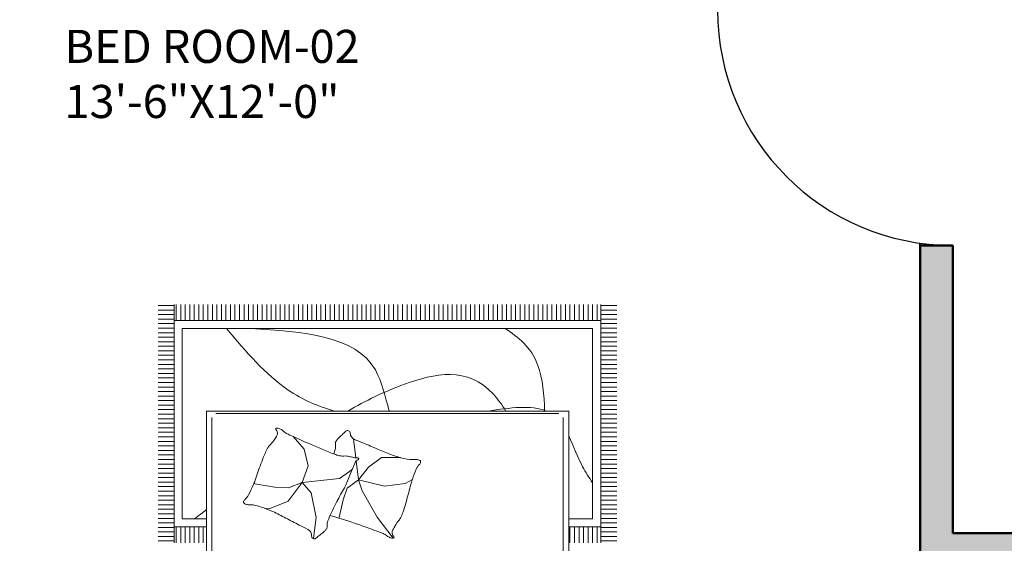
# Model space of a CAD drawing. Units: inches. Extents: x -7 to 1228, y -146 to 1091.
# Tile 22 of 88: x 664 to 815, y 113 to 194. Entities that reach past the tile are written whole.
import ezdxf

# ---------------------------------------------------------------- set-up
doc = ezdxf.new("R2010")
doc.units = ezdxf.units.IN
for name, color, linetype, lineweight in [('A-AREA-IDEN', 7, 'Continuous', 18), ('A-DOOR', 4, 'Continuous', 25), ('A-FURN', 8, 'Continuous', 18), ('A-WALL', 7, 'Continuous', 50), ('A-WALL-PATT', 251, 'Continuous', 13)]:
    doc.layers.add(name, color=color, linetype=linetype, lineweight=lineweight)
doc.styles.add('DIM_FONT', font='SIMPLEX.shx', dxfattribs={"width": 0.8})
doc.styles.get("Standard").update_dxf_attribs({"font": 'arial.ttf'})

# ---------------------------------------------------------------- blocks, each defined once
blk = doc.blocks.new('A$C4F634EDD')
for p, q in [((0.5, 0.5295), (0.5, 2.6295)), ((2.3, 2.6295), (2.3, 0.5295)), ((0.5258, 2.121), (0.5258, 0.5617)), ((2.2716, 0.5617), (2.2716, 1.7136)), ((0.2586, 1.1753), (0.3386, 1.1753)), ((0.3386, 0), (0.3386, 1.1852)), ((0.3486, 1.1052), (0.3486, 1.1852)), ((0.3711, 1.1052), (0.3711, 1.1852)), ((0.3936, 1.1052), (0.3936, 1.1852)), ((0.4161, 1.1052), (0.4161, 1.1852)), ((0.4386, 1.1052), (0.4386, 1.1852)), ((0.4611, 1.1052), (0.4611, 1.1852)), ((0.4836, 1.1052), (0.4836, 1.1852)), ((2.3061, 1.1052), (2.3061, 1.1852)), ((2.3286, 1.1052), (2.3286, 1.1852)), ((2.3511, 1.1052), (2.3511, 1.1852)), ((2.3736, 1.1052), (2.3736, 1.1852)), ((2.3961, 1.1052), (2.3961, 1.1852)), ((2.4186, 1.1052), (2.4186, 1.1852)), ((2.4411, 1.1052), (2.4411, 1.1852)), ((2.4588, 1.1852), (2.4588, 0)), ((2.4588, 1.1753), (2.5388, 1.1753)), ((0.2586, 1.1528), (0.3386, 1.1528)), ((0.2586, 1.1303), (0.3386, 1.1303)), ((1.031, 1.1612), (1.0448, 1.0581)), ((1.4276, 1.1611), (1.3484, 1.0571)), ((2.4588, 1.1528), (2.5388, 1.1528)), ((2.4588, 1.1303), (2.5388, 1.1303)), ((0.2586, 1.1078), (0.3386, 1.1078)), ((0.2586, 1.0853), (0.3386, 1.0853)), ((0.3386, 1.1052), (0.5, 1.1052)), ((2.3, 1.1052), (2.4588, 1.1052)), ((2.4588, 1.1078), (2.5388, 1.1078)), ((2.4588, 1.0853), (2.5388, 1.0853)), ((0.2586, 1.0628), (0.3386, 1.0628)), ((0.2586, 1.0403), (0.3386, 1.0403)), ((0.3786, 1.0652), (0.5, 1.0652)), ((0.3786, 0.12), (0.3786, 1.0652)), ((1.0448, 1.0581), (1.019, 0.936)), ((1.1784, 0.9702), (1.1586, 1.0591)), ((1.3484, 1.0571), (1.2733, 0.9268)), ((2.3, 1.0652), (2.4188, 1.0652)), ((2.4188, 1.0652), (2.4188, 0.12)), ((2.4588, 1.0628), (2.5388, 1.0628)), ((2.4588, 1.0403), (2.5388, 1.0403)), ((0.2586, 1.0178), (0.3386, 1.0178)), ((0.2586, 0.9953), (0.3386, 0.9953)), ((0.8108, 1.0151), (0.7868, 1.0117)), ((0.9054, 0.9773), (0.8108, 1.0151)), ((2.4588, 1.0178), (2.5388, 1.0178)), ((2.4588, 0.9953), (2.5388, 0.9953)), ((0.2586, 0.9728), (0.3386, 0.9728)), ((0.2586, 0.9503), (0.3386, 0.9503)), ((0.9743, 0.8845), (0.9054, 0.9773)), ((1.019, 0.936), (0.9743, 0.8845)), ((1.1982, 0.9129), (1.1784, 0.9702)), ((2.4588, 0.9728), (2.5388, 0.9728)), ((2.4588, 0.9503), (2.5388, 0.9503)), ((0.2586, 0.9278), (0.3386, 0.9278)), ((0.2586, 0.9053), (0.3386, 0.9053)), ((0.2586, 0.8828), (0.3386, 0.8828)), ((0.7403, 0.8913), (0.737, 0.8849)), ((0.8384, 0.9085), (0.7403, 0.8913)), ((0.9072, 0.912), (0.8384, 0.9085)), ((0.9743, 0.8845), (0.9072, 0.912)), ((0.9743, 0.8845), (1.0052, 0.802)), ((0.9743, 0.8845), (1.16, 0.8656)), ((1.1973, 0.8853), (1.2203, 0.829)), ((1.2555, 0.8715), (1.1982, 0.9129)), ((1.2733, 0.9268), (1.2555, 0.8715)), ((1.2555, 0.8715), (1.384, 0.9031)), ((1.384, 0.9031), (1.4868, 0.8892)), ((1.4868, 0.8892), (1.5228, 0.8692)), ((2.4588, 0.9278), (2.5388, 0.9278)), ((2.4588, 0.9053), (2.5388, 0.9053)), ((2.4588, 0.8828), (2.5388, 0.8828)), ((0.2586, 0.8603), (0.3386, 0.8603)), ((0.2586, 0.8378), (0.3386, 0.8378)), ((1.16, 0.8656), (1.2099, 0.8295)), ((1.2555, 0.8715), (1.2437, 0.7773)), ((1.2555, 0.8715), (1.3049, 0.8082)), ((2.4588, 0.8603), (2.5388, 0.8603)), ((2.4588, 0.8378), (2.5388, 0.8378)), ((0.2586, 0.8153), (0.3386, 0.8153)), ((0.2586, 0.7928), (0.3386, 0.7928)), ((1.0052, 0.802), (0.9846, 0.7194)), ((1.2099, 0.8295), (1.222, 0.8209)), ((1.2203, 0.829), (1.2381, 0.7855)), ((1.3049, 0.8082), (1.3701, 0.7608)), ((2.4588, 0.8153), (2.5388, 0.8153)), ((2.4588, 0.7928), (2.5388, 0.7928)), ((0.2586, 0.7703), (0.3386, 0.7703)), ((0.2586, 0.7478), (0.3386, 0.7478)), ((1.2419, 0.7626), (1.23, 0.668)), ((1.3701, 0.7608), (1.463, 0.7608)), ((2.4588, 0.7703), (2.5388, 0.7703)), ((2.4588, 0.7478), (2.5388, 0.7478)), ((0.2586, 0.7253), (0.3386, 0.7253)), ((0.2586, 0.7028), (0.3386, 0.7028)), ((0.9846, 0.7194), (0.931, 0.6569)), ((2.4588, 0.7253), (2.5388, 0.7253)), ((2.4588, 0.7028), (2.5388, 0.7028)), ((0.2586, 0.6803), (0.3386, 0.6803)), ((0.2586, 0.6578), (0.3386, 0.6578)), ((2.4588, 0.6803), (2.5388, 0.6803)), ((2.4588, 0.6578), (2.5388, 0.6578)), ((0.2586, 0.6353), (0.3386, 0.6353)), ((0.2586, 0.6128), (0.3386, 0.6128)), ((0.2586, 0.5903), (0.3386, 0.5903)), ((2.4588, 0.6353), (2.5388, 0.6353)), ((2.4588, 0.6128), (2.5388, 0.6128)), ((2.4588, 0.5903), (2.5388, 0.5903)), ((0.2586, 0.5678), (0.3386, 0.5678)), ((0.2586, 0.5453), (0.3386, 0.5453)), ((0.5458, 0.5417), (2.2516, 0.5417)), ((2.4588, 0.5678), (2.5388, 0.5678)), ((2.4588, 0.5453), (2.5388, 0.5453)), ((0.2586, 0.5228), (0.3386, 0.5228)), ((0.2586, 0.5003), (0.3386, 0.5003)), ((2.3, 0.5295), (0.5, 0.5295)), ((2.4588, 0.5228), (2.5388, 0.5228)), ((2.4588, 0.5003), (2.5388, 0.5003)), ((0.2586, 0.4778), (0.3386, 0.4778)), ((0.2586, 0.4553), (0.3386, 0.4553)), ((2.4588, 0.4778), (2.5388, 0.4778)), ((2.4588, 0.4553), (2.5388, 0.4553)), ((0.2586, 0.4328), (0.3386, 0.4328)), ((0.2586, 0.4103), (0.3386, 0.4103)), ((2.4588, 0.4328), (2.5388, 0.4328)), ((2.4588, 0.4103), (2.5388, 0.4103)), ((0.2586, 0.3878), (0.3386, 0.3878)), ((0.2586, 0.3653), (0.3386, 0.3653)), ((0.2586, 0.3428), (0.3386, 0.3428)), ((2.4588, 0.3878), (2.5388, 0.3878)), ((2.4588, 0.3653), (2.5388, 0.3653)), ((2.4588, 0.3428), (2.5388, 0.3428)), ((0.2586, 0.3203), (0.3386, 0.3203)), ((0.2586, 0.2978), (0.3386, 0.2978)), ((2.4588, 0.3203), (2.5388, 0.3203)), ((2.4588, 0.2978), (2.5388, 0.2978)), ((0.2586, 0.2753), (0.3386, 0.2753)), ((0.2586, 0.2528), (0.3386, 0.2528)), ((2.4588, 0.2753), (2.5388, 0.2753)), ((2.4588, 0.2528), (2.5388, 0.2528)), ((0.2586, 0.2303), (0.3386, 0.2303)), ((0.2586, 0.2078), (0.3386, 0.2078)), ((2.4588, 0.2303), (2.5388, 0.2303)), ((2.4588, 0.2078), (2.5388, 0.2078)), ((0.2586, 0.1853), (0.3386, 0.1853)), ((0.2586, 0.1628), (0.3386, 0.1628)), ((2.4588, 0.1853), (2.5388, 0.1853)), ((2.4588, 0.1628), (2.5388, 0.1628)), ((0.2586, 0.1403), (0.3386, 0.1403)), ((0.2586, 0.1178), (0.3386, 0.1178)), ((2.4188, 0.12), (0.3786, 0.12)), ((2.4588, 0.1403), (2.5388, 0.1403)), ((2.4588, 0.1178), (2.5388, 0.1178)), ((0.2586, 0.0953), (0.3386, 0.0953)), ((0.2586, 0.0728), (0.3386, 0.0728)), ((0.2586, 0.0503), (0.3386, 0.0503)), ((2.4588, 0.08), (0.3386, 0.08)), ((0.3486, 0), (0.3486, 0.08)), ((0.3711, 0), (0.3711, 0.08)), ((0.3936, 0), (0.3936, 0.08)), ((0.4161, 0), (0.4161, 0.08)), ((0.4386, 0), (0.4386, 0.08)), ((0.4611, 0), (0.4611, 0.08)), ((0.4836, 0), (0.4836, 0.08)), ((0.5061, 0), (0.5061, 0.08)), ((0.5286, 0), (0.5286, 0.08)), ((0.5511, 0), (0.5511, 0.08)), ((0.5736, 0), (0.5736, 0.08)), ((0.5961, 0), (0.5961, 0.08)), ((0.6186, 0), (0.6186, 0.08)), ((0.6411, 0), (0.6411, 0.08)), ((0.6636, 0), (0.6636, 0.08)), ((0.6861, 0), (0.6861, 0.08)), ((0.7086, 0), (0.7086, 0.08)), ((0.7311, 0), (0.7311, 0.08)), ((0.7536, 0), (0.7536, 0.08)), ((0.7761, 0), (0.7761, 0.08)), ((0.7986, 0), (0.7986, 0.08)), ((0.8211, 0), (0.8211, 0.08)), ((0.8436, 0), (0.8436, 0.08)), ((0.8661, 0), (0.8661, 0.08)), ((0.8886, 0), (0.8886, 0.08)), ((0.9111, 0), (0.9111, 0.08)), ((0.9336, 0), (0.9336, 0.08)), ((0.9561, 0), (0.9561, 0.08)), ((0.9786, 0), (0.9786, 0.08)), ((1.0011, 0), (1.0011, 0.08)), ((1.0236, 0), (1.0236, 0.08)), ((1.0461, 0), (1.0461, 0.08)), ((1.0686, 0), (1.0686, 0.08)), ((1.0911, 0), (1.0911, 0.08)), ((1.1136, 0), (1.1136, 0.08)), ((1.1361, 0), (1.1361, 0.08)), ((1.1586, 0), (1.1586, 0.08)), ((1.1811, 0), (1.1811, 0.08)), ((1.2036, 0), (1.2036, 0.08)), ((1.2261, 0), (1.2261, 0.08)), ((1.2486, 0), (1.2486, 0.08)), ((1.2711, 0), (1.2711, 0.08)), ((1.2936, 0), (1.2936, 0.08)), ((1.3161, 0), (1.3161, 0.08)), ((1.3386, 0), (1.3386, 0.08)), ((1.3611, 0), (1.3611, 0.08)), ((1.3836, 0), (1.3836, 0.08)), ((1.4061, 0), (1.4061, 0.08)), ((1.4286, 0), (1.4286, 0.08)), ((1.4511, 0), (1.4511, 0.08)), ((1.4736, 0), (1.4736, 0.08)), ((1.4961, 0), (1.4961, 0.08)), ((1.5186, 0), (1.5186, 0.08)), ((1.5411, 0), (1.5411, 0.08)), ((1.5636, 0), (1.5636, 0.08)), ((1.5861, 0), (1.5861, 0.08)), ((1.6086, 0), (1.6086, 0.08)), ((1.6311, 0), (1.6311, 0.08)), ((1.6536, 0), (1.6536, 0.08)), ((1.6761, 0), (1.6761, 0.08)), ((1.6986, 0), (1.6986, 0.08)), ((1.7211, 0), (1.7211, 0.08)), ((1.7436, 0), (1.7436, 0.08)), ((1.7661, 0), (1.7661, 0.08)), ((1.7886, 0), (1.7886, 0.08)), ((1.8111, 0), (1.8111, 0.08)), ((1.8336, 0), (1.8336, 0.08)), ((1.8561, 0), (1.8561, 0.08)), ((1.8786, 0), (1.8786, 0.08)), ((1.9011, 0), (1.9011, 0.08)), ((1.9236, 0), (1.9236, 0.08)), ((1.9461, 0), (1.9461, 0.08)), ((1.9686, 0), (1.9686, 0.08)), ((1.9911, 0), (1.9911, 0.08)), ((2.0136, 0), (2.0136, 0.08)), ((2.0361, 0), (2.0361, 0.08)), ((2.0586, 0), (2.0586, 0.08)), ((2.0811, 0), (2.0811, 0.08)), ((2.1036, 0), (2.1036, 0.08)), ((2.1261, 0), (2.1261, 0.08)), ((2.1486, 0), (2.1486, 0.08)), ((2.1711, 0), (2.1711, 0.08)), ((2.1936, 0), (2.1936, 0.08)), ((2.2161, 0), (2.2161, 0.08)), ((2.2386, 0), (2.2386, 0.08)), ((2.2611, 0), (2.2611, 0.08)), ((2.2836, 0), (2.2836, 0.08)), ((2.3061, 0), (2.3061, 0.08)), ((2.3286, 0), (2.3286, 0.08)), ((2.3511, 0), (2.3511, 0.08)), ((2.3736, 0), (2.3736, 0.08)), ((2.3961, 0), (2.3961, 0.08)), ((2.4186, 0), (2.4186, 0.08)), ((2.4411, 0), (2.4411, 0.08)), ((2.4588, 0.0953), (2.5388, 0.0953)), ((2.4588, 0.0728), (2.5388, 0.0728)), ((2.4588, 0.0503), (2.5388, 0.0503)), ((0.2586, 0.0278), (0.3386, 0.0278)), ((0.2586, 0.0053), (0.3386, 0.0053)), ((2.4588, 0.0278), (2.5388, 0.0278)), ((2.4588, 0.0053), (2.5388, 0.0053))]:
    blk.add_line(p, q)
for centre, radius, start, end in [((0.9863, 1.1494), 0.0359, 297.2902, 3.2455), ((1.0348, 1.1521), 0.0127, 51.1864, 183.2455), ((0.9991, 1.1077), 0.0697, 45.8726, 51.1864), ((1.0791, 1.1902), 0.0452, 225.8726, 232.4713), ((1.2846, 1.4577), 0.3825, 232.4713, 233.7837), ((0.6683, 0.6162), 0.6605, 52.7849, 53.7837), ((0.9362, 0.9689), 0.2176, 46.4776, 52.7849), ((1.0327, 1.0706), 0.0774, 35.8936, 46.4776), ((1.0543, 1.9106), 0.8371, 290.1287, 292.7069), ((1.3469, 1.2115), 0.0792, 292.7069, 308.5854), ((1.4338, 1.1026), 0.0601, 110.3452, 128.5854), ((1.4251, 1.1259), 0.0352, 86.0516, 110.3452), ((1.4996, 1.1284), 0.0771, 169.5926, 177.2714), ((1.4378, 1.1314), 0.0153, 177.2714, 194.5709), ((1.4611, 1.1374), 0.0393, 194.5709, 206.8179), ((1.4376, 1.1398), 0.0142, 126.5792, 169.5926), ((1.4273, 1.1567), 0.00443, 13.2808, 86.0516), ((1.4254, 1.1562), 0.0063, 306.5792, 13.2808), ((3.744, -4.3336), 6.1019, 117.49986, 117.84822), ((1.8575, -0.7096), 2.0162, 116.4147, 117.4999), ((-0.4173, 3.8699), 3.0972, 296.4147, 297.2902), ((1.0771, 1.1027), 0.0226, 351.9508, 35.8936), ((1.1449, 1.0931), 0.0458, 171.9508, 202.4162), ((0.2266, 4.0657), 3.145, 286.6085, 289.0836), ((-0.4107, 5.9078), 5.0942, 289.0836, 290.1287), ((1.7401, 1.2785), 0.352, 206.8179, 210.9056), ((1.6045, 1.1973), 0.194, 210.9056, 219.7005), ((0.5736, 1.5979), 0.6236, 290.7486, 297.4921), ((-1.8336, 6.2238), 5.8383, 297.49208, 297.84822), ((2.032, 1.4591), 1.0054, 202.4162, 205.0529), ((1.0922, 1.1636), 0.1166, 280.7366, 286.6085), ((2.6493, 1.7476), 1.6868, 205.0529, 207.0884), ((1.3929, 1.0217), 0.081, 26.0735, 39.7005), ((1.2892, 0.9709), 0.1965, 17.8396, 26.0735), ((-0.4304, 0.4175), 2.003, 15.2625, 17.8396), ((0.6894, 0.9832), 0.0058, 121.6917, 179.0386), ((0.7004, 0.983), 0.0168, 179.0386, 229.4914), ((0.7131, 0.9448), 0.0509, 103.0402, 121.6917), ((0.7152, 0.9361), 0.0599, 86.6119, 103.0402), ((0.7224, 1.0587), 0.063, 266.6119, 282.6252), ((0.6422, 1.4168), 0.43, 282.6252, 290.7486), ((2.541, 1.6922), 1.5652, 207.0884, 209.936), ((0.6405, 0.9128), 0.0755, 26.3332, 49.4914), ((-1.6775, -0.2344), 2.6619, 25.1732, 26.3332), ((-0.0881, 0.5109), 1.6481, 13.841, 15.2625), ((0.5689, 0.8213), 0.1798, 20.7081, 25.1732), ((0.2268, 0.692), 0.5454, 18.2369, 20.7081), ((0.9989, 0.8042), 0.2143, 22.2355, 29.936), ((2.0418, 1.0357), 0.5454, 193.841, 196.3122), ((1.6908, 0.933), 0.1798, 196.3122, 200.7773), ((2.3102, 1.3785), 1.6481, 198.2369, 199.6584), ((4.0115, 1.8135), 2.6619, 200.7773, 201.9373), ((2.6444, 1.4979), 2.003, 199.6584, 202.2355), ((1.2594, 0.7942), 0.0231, 202.2355, 252.8133), ((1.6124, 0.8472), 0.0755, 201.9373, 225.0955), ((1.5473, 0.7819), 0.0168, 354.6428, 45.0955), ((0.9722, 0.8143), 0.1965, 202.2355, 210.4694), ((2.2689, -2.1899), 3.145, 111.0043, 113.4795), ((0.1831, 0.4093), 1.0054, 18.0203, 19.3448), ((1.1834, 0.6373), 0.1166, 98.1216, 111.0043), ((1.1763, 0.687), 0.0663, 85.4882, 98.1216), ((1.1871, 0.8241), 0.0712, 265.4882, 277.6784), ((1.1727, 0.9313), 0.1794, 277.6784, 284.8807), ((1.2689, 0.569), 0.1955, 97.9822, 104.8807), ((1.2465, 0.729), 0.034, 85.7407, 97.9822), ((1.2497, 0.772), 0.0092, 265.7407, 289.3799), ((1.2512, 0.7678), 0.00467, 289.3799, 72.8133), ((1.6266, 0.159), 0.6236, 106.3527, 113.0962), ((1.5721, 0.3449), 0.43, 98.2293, 106.3527), ((1.5195, 0.708), 0.063, 82.216, 98.2293), ((1.5362, 0.8298), 0.0599, 262.216, 278.6443), ((1.5375, 0.8209), 0.0509, 278.6443, 297.2959), ((1.5582, 0.7808), 0.0058, 297.2959, 354.6428), ((0.8727, 0.7557), 0.081, 210.4694, 224.0964), ((0.6752, 0.5644), 0.194, 35.3015, 44.0964), ((3.0455, -3.9778), 5.0942, 113.4795, 114.5246), ((1.0957, 0.7061), 0.0458, 347.5549, 18.0203), ((1.1625, 0.6914), 0.0226, 167.5549, 211.4977), ((2.4404, -2.1823), 3.0972, 112.0188, 112.8944), ((0.5234, 2.5582), 2.0162, 292.0188, 293.104), ((-1.0798, 6.3161), 6.1019, 293.10398, 293.45234), ((3.6722, -4.6377), 5.8383, 113.0962, 113.45234), ((0.5462, 0.4731), 0.352, 31.2138, 35.3015), ((0.8136, 0.6351), 0.0393, 18.9668, 31.2138), ((0.8364, 0.6429), 0.0153, 1.6673, 18.9668), ((0.7746, 0.6411), 0.0771, 353.9885, 1.6673), ((0.9332, 0.57), 0.0792, 117.1028, 132.9813), ((1.2784, -0.1047), 0.8371, 114.5246, 117.1028), ((1.2092, 0.72), 0.0774, 211.4977, 222.0817), ((1.3133, 0.814), 0.2176, 222.0817, 228.389), ((1.6074, 1.1451), 0.6605, 228.389, 229.3878), ((0.9284, 0.3533), 0.3825, 48.0754, 49.3878), ((1.1538, 0.6043), 0.0452, 41.4767, 48.0754), ((1.2009, 0.6389), 0.0127, 226.7905, 358.8496), ((1.2495, 0.6379), 0.0359, 112.8944, 178.8496), ((0.8506, 0.6191), 0.0063, 130.9751, 197.6767), ((0.8488, 0.6185), 0.00443, 197.6767, 270.4475), ((0.8372, 0.6345), 0.0142, 310.9751, 353.9885), ((0.8486, 0.6493), 0.0352, 270.4475, 294.7411), ((0.8382, 0.6719), 0.0601, 294.7411, 312.9813), ((1.2399, 0.6804), 0.0697, 221.4767, 226.7905)]:
    blk.add_arc(centre, radius, start, end)
for points in [[(0.4393, 1.0652), (0.4595, 1.05), (0.4798, 1.0348), (0.5, 1.0195)], [(1.9003, 0.5295), (2.0065, 0.514), (2.1132, 0.4978), (2.1894, 0.5295)]]:
    blk.add_open_spline(points, degree=3)
for points, knots in [([(2.3, 0.6535), (2.3236, 0.7026), (2.3554, 0.7914), (2.4015, 0.8608), (2.4188, 0.8868)], [1893.525221, 1893.525221, 1893.525221, 1893.525221, 2051.902476, 2146.74457, 2146.74457, 2146.74457, 2146.74457]), ([(0.5992, 0.12), (0.6957, 0.2341), (0.8523, 0.4189), (1.0536, 0.5069), (1.136, 0.5295)], [0, 0, 0, 0, 432.822832, 701.445452, 701.445452, 701.445452, 701.445452]), ([(0.7187, 0.12), (0.9791, 0.1362), (1.326, 0.1577), (1.3868, 0.4574), (1.408, 0.5295)], [0, 0, 0, 0, 653.160442, 870.050857, 870.050857, 870.050857, 870.050857]), ([(1.2016, 0.5295), (1.2892, 0.479), (1.5144, 0.3684), (1.8265, 0.2994), (1.9681, 0.4992), (1.9875, 0.5295)], [936.534237, 936.534237, 936.534237, 936.534237, 1243.285375, 1683.261222, 1758.254386, 1758.254386, 1758.254386, 1758.254386]), ([(2.1796, 0.5295), (2.1798, 0.4519), (2.1548, 0.2369), (2.0487, 0.164), (1.9846, 0.12)], [2202.034493, 2202.034493, 2202.034493, 2202.034493, 2357.807635, 2594.446174, 2594.446174, 2594.446174, 2594.446174])]:
    blk.add_open_spline(points, degree=3, knots=knots)
at = {"style": 'DIM_FONT', "width": 0.8, "flags": 9}
for tag, p in [('YSIZE', (0.5, 2.6295)), ('XSIZE', (0.5, 2.6295)), ('XSIZE', (2.2985, 2.6295)), ('YSIZE', (2.2985, 2.6295))]:
    blk.add_attdef(tag, p, '', height=0.0005, dxfattribs=at)
blk = doc.blocks.new('DOOR-900')
blk.add_line((36, 0), (36, 36))
blk.add_arc((36, 0), 36, 90, 180)

msp = doc.modelspace()

# ---------------------------------------------------------------- hatches: boundary and pattern name
at = {"layer": 'A-WALL-PATT'}
h = msp.add_hatch(color=256, dxfattribs=at)
h.dxf.hatch_style = 1
h.paths.add_polyline_path([(69, 568), (60, 568), (60, 493), (63.29, 493), (69, 493)])
h.paths.add_polyline_path([(69, 662.41), (60, 662.41), (60, 586), (69, 586)], flags=17)
h.paths.add_polyline_path([(69, 723), (184, 723), (184, 734), (179, 734), (179, 728), (69, 728), (69, 741.62), (60, 741.62), (60, 698.41), (69, 698.41)], flags=17)
h.paths.add_polyline_path([(69, 782), (231, 782), (231, 728), (231, 723), (231, 586), (236, 586), (236, 787), (69, 787), (69, 800.13), (60, 800.13), (60, 765.62), (69, 765.62)])
h.paths.add_polyline_path([(184, 842), (189, 842), (189, 848), (173, 848), (173, 842), (179, 842), (179, 787), (184, 787)])
h.paths.add_polyline_path([(118.22, 69), (69, 69), (69, 60), (118.22, 60)])
h.paths.add_polyline_path([(227, 69), (154.22, 69), (154.22, 60), (227, 60)])
h.paths.add_polyline_path([(236, 60), (232.71, 60), (227, 60), (227, 36), (236, 36)])
h.paths.add_polyline_path([(389, 60), (380, 60), (380, 36), (389, 36)])
h.paths.add_polyline_path([(384, 181), (380, 181), (380, 115), (380, 78), (384, 78)])
h.paths.add_polyline_path([(380, 115), (334.55, 115), (334.55, 109), (380, 109)])
h.paths.add_polyline_path([(274.55, 115), (236, 115), (236, 201), (232.71, 201), (231, 201), (231, 78), (236, 78), (236, 109), (274.55, 109)])
h.paths.add_polyline_path([(69, 123), (60, 123), (60, 78), (69, 78)])
h.paths.add_polyline_path([(69, 201), (60, 201), (60, 159), (69, 159)])
h.paths.add_polyline_path([(143, 219), (69, 219), (69, 213), (143, 213)], flags=17)
h.paths.add_polyline_path([(189, 219), (184, 219), (184, 274), (231, 274), (231, 219), (236, 219), (236, 279), (184, 279), (184, 297), (179, 297), (179, 279), (69, 279), (69, 290.91), (60, 290.91), (60, 262.18), (69, 262.18), (69, 274), (179, 274), (179, 219), (173, 219), (173, 213), (189, 213)])
h.paths.add_polyline_path([(69, 238.18), (60, 238.18), (60, 219), (69, 219)], flags=17)
h.paths.add_polyline_path([(69, 333), (60, 333), (60, 314.91), (69, 314.91), (69, 316.96)])
h.paths.add_polyline_path([(190, 338), (184, 338), (69, 338), (69, 333), (179, 333), (179, 327), (184, 327), (184, 333.02), (190, 333.05)])
h.paths.add_polyline_path([(69, 386.81), (60, 386.81), (60, 351), (69, 351)])
h.paths.add_polyline_path([(69, 475), (60, 475), (60, 422.81), (69, 422.81)])
h.paths.add_polyline_path([(236, 475), (231, 475), (231, 351.24), (236, 351.24)])
h.paths.add_polyline_path([(384, 475), (380, 475), (380, 362), (384, 362)])
h.paths.add_polyline_path([(547, 307), (439, 307), (439, 356), (445, 356), (445, 362), (433, 362), (433, 307), (380, 307), (380, 244), (380, 241), (384, 241), (384, 301), (433, 301), (433, 277), (439, 277), (439, 301), (547, 301)])
h.paths.add_polyline_path([(547, 241), (439, 241), (439, 247), (433, 247), (433, 235), (547, 235)])
h.paths.add_polyline_path([(450, 69), (440.29, 69), (424.89, 69), (389, 69), (389, 60), (450, 60)])
h.paths.add_polyline_path([(547, 69), (486, 69), (486, 60), (547, 60)])
h.paths.add_polyline_path([(556, 148.27), (547, 148.27), (547, 78), (556, 78)])
h.paths.add_polyline_path([(556, 223), (547, 223), (547, 195), (547, 184.27), (556, 184.27)])
h.paths.add_polyline_path([(556, 311.19), (547, 311.19), (547, 273.08), (556, 273.08)])
h.paths.add_polyline_path([(556, 344), (552.71, 344), (547, 344), (547, 335.19), (556, 335.19)])
h.paths.add_polyline_path([(556, 249.08), (547, 249.08), (547, 241), (556, 241)])
h.paths.add_polyline_path([(547, 362), (475, 362), (475, 356), (547, 356)], flags=0)
h.paths.add_polyline_path([(556, 399.62), (547, 399.62), (547, 362), (556, 362)])
h.paths.add_polyline_path([(556, 475), (547, 475), (547, 435.62), (556, 435.62)])
h.paths.add_polyline_path([(547, 493), (389, 493), (389, 487), (547, 487)])
h.paths.add_polyline_path([(380, 493), (278, 493), (278, 487), (380, 487)])
h.paths.add_polyline_path([(227, 493), (69, 493), (69, 487), (227, 487)])
h.paths.add_polyline_path([(643, 122.44), (634, 122.44), (634, 78), (643, 78)])
h.paths.add_polyline_path([(702.5, 69), (692.79, 69), (677.39, 69), (643, 69), (643, 60), (702.5, 60)])
h.paths.add_polyline_path([(798, 69), (738.5, 69), (738.5, 60), (798, 60)])
h.paths.add_polyline_path([(807, 60), (803.71, 60), (798, 60), (798, 36), (807, 36)])
h.paths.add_polyline_path([(807, 109), (846.75, 109), (846.75, 115), (807, 115), (807, 159), (802, 159), (802, 78), (807, 78)])
h.paths.add_polyline_path([(807, 201), (802, 201), (802, 195), (807, 195)])
h.paths.add_polyline_path([(643, 201), (634, 201), (634, 158.44), (643, 158.44)])
h.paths.add_polyline_path([(756, 225), (751, 225), (751, 219), (643, 219), (643, 213), (756, 213)])
h.paths.add_polyline_path([(643, 240.85), (634, 240.85), (634, 219), (643, 219)])
h.paths.add_polyline_path([(643, 274), (643, 288.63), (634, 288.63), (634, 264.85), (643, 264.85)])
h.paths.add_polyline_path([(802, 279), (756, 279), (756, 297), (751, 297), (751, 279), (643, 279), (643, 274), (751, 274), (751, 255), (756, 255), (756, 274), (802, 274)])
h.paths.add_polyline_path([(807, 333), (803.71, 333), (802, 333), (802, 279), (802, 274), (802, 219), (807, 219)])
h.paths.add_polyline_path([(956, 182), (951, 182), (951, 115), (906.75, 115), (906.75, 109), (951, 109), (951, 78), (956, 78)])
h.paths.add_polyline_path([(960, 60), (951, 60), (951, 36), (960, 36)])
h.paths.add_polyline_path([(1021, 69), (1005.78, 69), (960, 69), (960, 60), (1021, 60)])
h.paths.add_polyline_path([(956, 224), (951, 224), (951, 218), (956, 218)])
h.paths.add_polyline_path([(956, 302), (1004, 302), (1004, 278), (1010, 278), (1010, 302), (1118, 302), (1118, 290.81), (1127, 290.81), (1127, 326.97), (1118, 326.97), (1118, 320.97), (1118, 307), (1010, 307), (1010, 356), (1016, 356), (1016, 362), (1004, 362), (1004, 307), (951, 307), (951, 244), (951, 242), (954.29, 242), (956, 242)])
h.paths.add_polyline_path([(643, 333), (634, 333), (634, 312.63), (643, 312.63), (643, 316.96)])
h.paths.add_polyline_path([(756, 338), (643, 338), (643, 333), (751, 333), (751, 327), (756, 327)])
h.paths.add_polyline_path([(643, 388), (634, 388), (634, 351), (643, 351)])
h.paths.add_polyline_path([(807, 357), (802, 357), (802, 351), (807, 351)])
h.paths.add_polyline_path([(807, 475), (802, 475), (802, 393), (807, 393)])
h.paths.add_polyline_path([(643, 475), (634, 475), (634, 424), (643, 424)])
h.paths.add_polyline_path([(798, 493), (643, 493), (643, 487), (798, 487)])
h.paths.add_polyline_path([(634, 493), (556, 493), (556, 487), (634, 487)])
h.paths.add_polyline_path([(813, 493), (807, 493), (807, 487), (813, 487)])
h.paths.add_polyline_path([(951, 493), (849, 493), (849, 487), (951, 487)])
h.paths.add_polyline_path([(956, 484), (951, 484), (951, 374), (956, 374)])
h.paths.add_polyline_path([(1109, 493), (969, 493), (969, 487), (1109, 487)])
h.paths.add_polyline_path([(1127, 484), (1118, 484), (1118, 450.64), (1127, 450.64)])
h.paths.add_polyline_path([(1127, 414.64), (1118, 414.64), (1118, 365), (1127, 365)])
h.paths.add_polyline_path([(1109, 362), (1046, 362), (1046, 356), (1109, 356)], flags=17)
h.paths.add_polyline_path([(1127, 356), (1123.45, 356), (1118, 356), (1118, 350.97), (1127, 350.97)], flags=0)
h.paths.add_polyline_path([(1127, 266.81), (1118, 266.81), (1118, 262.36), (1118, 242), (1127, 242)], flags=17)
h.paths.add_polyline_path([(1118, 242), (1010, 242), (1010, 248), (1004, 248), (1004, 237), (1118, 237)])
h.paths.add_polyline_path([(1127, 224), (1118, 224), (1118, 170), (1127, 170)])
h.paths.add_polyline_path([(1127, 134), (1118, 134), (1118, 78), (1127, 78)])
h.paths.add_polyline_path([(1118, 69), (1057, 69), (1057, 60), (1118, 60)])
h.paths.add_polyline_path([(227, 571.55), (227, 574), (69, 574), (69, 568), (227, 568)])
h.paths.add_polyline_path([(380, 571.55), (380, 574), (278, 574), (278, 568), (380, 568)])
h.paths.add_polyline_path([(242, 574), (236, 574), (236, 568), (242, 568)])
h.paths.add_polyline_path([(547, 571.55), (547, 574), (389, 574), (389, 568), (547, 568)])
h.paths.add_polyline_path([(384, 733), (380, 733), (380, 586), (384, 586)])
h.paths.add_polyline_path([(556, 646), (634, 646), (634, 655), (547, 655), (547, 586), (556, 586)])
h.paths.add_polyline_path([(634, 574), (556, 574), (556, 568), (634, 568)])
h.paths.add_polyline_path([(643, 655), (634, 655), (634, 586), (643, 586)])
h.paths.add_polyline_path([(798, 574), (643, 574), (643, 568), (798, 568)])
h.paths.add_polyline_path([(643, 663.85), (634, 663.85), (634, 655), (643, 655)])
h.paths.add_polyline_path([(556, 676.97), (547, 676.97), (547, 655), (556, 655)])
h.paths.add_polyline_path([(556, 733), (547, 733), (547, 712.97), (556, 712.97)])
h.paths.add_polyline_path([(643, 710), (634, 710), (634, 699.85), (643, 699.85)])
h.paths.add_polyline_path([(807, 668), (802, 668), (802, 586), (807, 586)])
h.paths.add_polyline_path([(951, 574), (849, 574), (849, 568), (951, 568)])
h.paths.add_polyline_path([(956, 691), (951, 691), (951, 577), (956, 577)])
h.paths.add_polyline_path([(1109, 574), (969, 574), (969, 568), (1109, 568)])
h.paths.add_polyline_path([(1127, 643.4), (1118, 643.4), (1118, 577), (1127, 577)])
h.paths.add_polyline_path([(1127, 568), (1123.45, 568), (1118, 568), (1118, 493), (1127, 493)])
h.paths.add_polyline_path([(1127, 733), (1118, 733), (1118, 679.4), (1127, 679.4)])
h.paths.add_polyline_path([(1127, 777.35), (1118, 777.35), (1118, 770.04), (1118, 751), (1127, 751)], flags=17)
h.paths.add_polyline_path([(1118, 751), (1010, 751), (1010, 757), (1004, 757), (1004, 745), (1118, 745)])
h.paths.add_polyline_path([(956, 811), (1004, 811), (1004, 787), (1010, 787), (1010, 811), (1017.87, 811), (1017.87, 811.63, -0.414214), (1018.25, 812), (1031.98, 812, -0.414214), (1032.35, 811.63), (1032.35, 811), (1118, 811), (1118, 801.35), (1127, 801.35), (1127, 834.69), (1118, 834.69), (1118, 830.24), (1118, 817), (1010, 817), (1010, 866), (1016, 866), (1016, 872), (1004, 872), (1004, 817), (956, 817), (956, 866), (951, 866), (951, 751), (954.29, 751), (956, 751)])
h.paths.add_polyline_path([(1118, 872), (1046, 872), (1046, 866), (1118, 866)], flags=17)
h.paths.add_polyline_path([(1127, 924.71), (1118, 924.71), (1118, 884), (1127, 884)])
h.paths.add_polyline_path([(1127, 866), (1123.71, 866), (1118, 866), (1118, 858.69), (1127, 858.69)], flags=17)
h.paths.add_polyline_path([(956, 983), (951, 983), (951, 952), (807, 952), (807, 983), (802, 983), (802, 902), (807, 902), (807, 946), (951, 946), (951, 884), (956, 884)])
h.paths.add_polyline_path([(807, 842), (802, 842), (802, 787), (756, 787), (756, 806), (751, 806), (751, 787), (643, 787), (643, 782), (751, 782), (751, 764), (756, 764), (756, 782), (802, 782), (802, 728), (807, 728)])
h.paths.add_polyline_path([(756, 848), (643, 848), (643, 842), (751, 842), (751, 836), (756, 836)])
h.paths.add_polyline_path([(756, 734), (751, 734), (751, 728), (643, 728), (643, 723), (756, 723)])
h.paths.add_polyline_path([(643, 749.79), (634, 749.79), (634, 728), (637.29, 728), (643, 728)])
h.paths.add_polyline_path([(643, 805.41), (634, 805.41), (634, 773.79), (643, 773.79)])
h.paths.add_polyline_path([(643, 896.66), (634, 896.66), (634, 860), (637.29, 860), (643, 860)])
h.paths.add_polyline_path([(643, 842), (634, 842), (634, 829.41), (643, 829.41)])
h.paths.add_polyline_path([(643, 983), (634, 983), (634, 932.66), (643, 932.66)])
h.paths.add_polyline_path([(1127, 983), (1118, 983), (1118, 960.71), (1127, 960.71)])
h.paths.add_polyline_path([(1118, 1001), (1077.53, 1001), (1077.53, 992), (1118, 992)])
h.paths.add_polyline_path([(1041.53, 1001), (960, 1001), (960, 992), (1041.53, 992)])
h.paths.add_polyline_path([(960, 1025), (951, 1025), (951, 1001), (954.29, 1001), (960, 1001)])
h.paths.add_polyline_path([(807, 1025), (798, 1025), (798, 1001), (807, 1001)])
h.paths.add_polyline_path([(798, 1001), (738.5, 1001), (738.5, 992), (798, 992)])
h.paths.add_polyline_path([(702.5, 1001), (643, 1001), (643, 992), (702.5, 992)])
h.paths.add_polyline_path([(547, 1001), (499.11, 1001), (499.11, 992), (547, 992)])
h.paths.add_polyline_path([(463.11, 1001), (389, 1001), (389, 992), (463.11, 992)])
h.paths.add_polyline_path([(389, 1025), (380, 1025), (380, 1022), (380, 1001), (383.29, 1001), (389, 1001)])
h.paths.add_polyline_path([(236, 1025), (227, 1025), (227, 1001), (236, 1001)])
h.paths.add_polyline_path([(236, 983), (231, 983), (231, 860), (236, 860)])
h.paths.add_polyline_path([(274.55, 952), (236, 952), (236, 946), (274.55, 946)])
h.paths.add_polyline_path([(380, 952), (334.55, 952), (334.55, 946), (380, 946)])
h.paths.add_polyline_path([(384, 983), (380, 983), (380, 884), (383.29, 884), (384, 884)])
h.paths.add_polyline_path([(227, 1001), (155.01, 1001), (155.01, 992), (162.87, 992), (227, 992)])
h.paths.add_polyline_path([(119.01, 1001), (69, 1001), (69, 992), (119.01, 992)])
h.paths.add_polyline_path([(69, 983), (60, 983), (60, 922.99), (69, 922.99)])
h.paths.add_polyline_path([(69, 886.99), (60, 886.99), (60, 860), (63.29, 860), (69, 860)])
h.paths.add_polyline_path([(143, 848), (69, 848), (69, 842), (143, 842)])

# ---------------------------------------------------------------- linework, layer by layer
at = {"layer": 'A-WALL'}
for p, q in [((802, 159.35), (802, 60)), ((802, 60), (802, 159)), ((807, 159), (802, 159)), ((807, 115), (807, 159)), ((807, 159), (807, 115)), ((951, 115), (807, 115))]:
    msp.add_line(p, q, dxfattribs=at)

# ---------------------------------------------------------------- block references
at = {"layer": 'A-DOOR', "rotation": 89.99999999999969}
msp.add_blockref('DOOR-900', (807, 159), dxfattribs=at)
at = {"layer": 'A-FURN', "xscale": -30.79356024027943, "yscale": 30.79356024027943, "zscale": 30.79356024027943, "rotation": 180}
msp.add_blockref('A$C4F634EDD', (677.39, 149.97), dxfattribs=at)

# ---------------------------------------------------------------- texts
at = {"layer": 'A-AREA-IDEN', "insert": (671.04, 191.98), "char_height": 5.0568, "attachment_point": 1}
msp.add_mtext_dynamic_manual_height_columns('BED ROOM-02\\P13\'-6"X12\'-0"', width=137.2821, gutter_width=25.28, heights=[0], dxfattribs=at)

doc.saveas('drawing.dxf')
